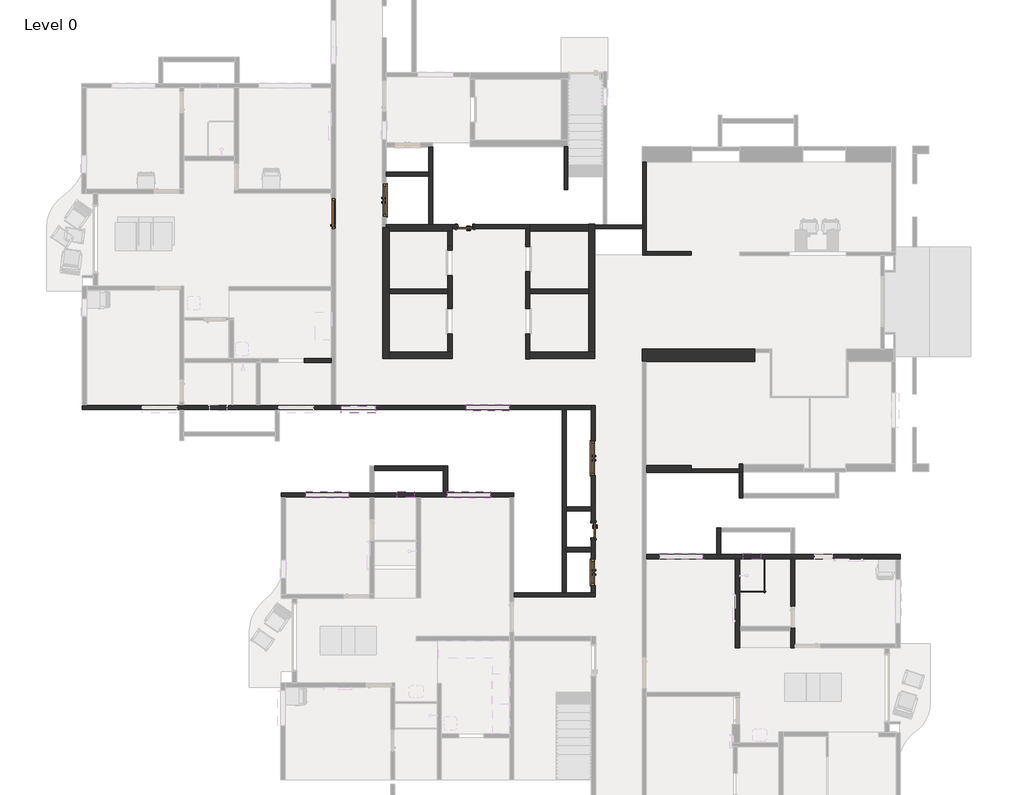
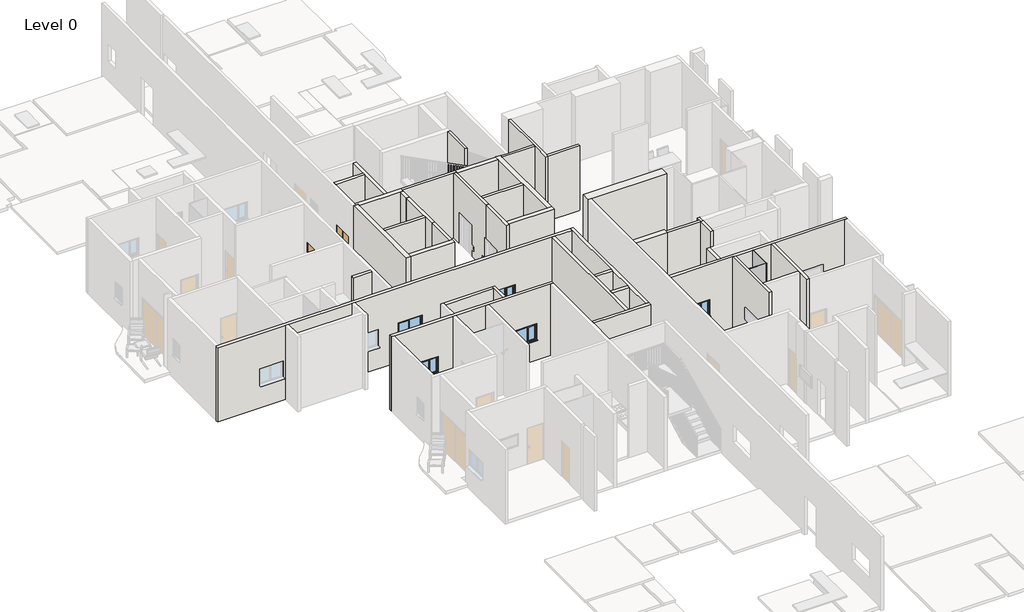
# One storey, part 5 of 14: 39 walls, 7 windows, 6 doors, 2 plates.
# Revit data of these elements (continued)
# Type "Windows_Concept_Plain_Dbl : 4'" (continued)
#   Rough Height = 910 mm
#   Height = 910 mm
#   Width = 1219.2 mm
#   Heat Transfer Coefficient (U) = 3.6886 W/(m²·K)
#   FrameOffset - External = 50 mm
#   Default Head Height = 2110 mm
#   Vis - Cavity Closers = yes
#   Define Thermal Properties by = 1
#   Material Trim = Window Frame
#   Material Glass = Glass
#   Material Frame = Window Frame
#   Wall Closure = (empty or 0)
# Type "Windows_Sgl_Plain : 2'"
#   Type Mark = "72"
#   Operation = "SinglePanel"
#   Construction Type Id = "SGL"
#   Manufacturer = "Revit"
#   Keynote = "L10"
#   Analytic Construction = "Large single-glazed windows"
#   Wrap Layers (Ext) from Ext = 102.5 mm
#   Wrap Layers (Int) from Ext = 177.5 mm
#   Window Board Projection = 25 mm
#   Window Board Extension = 25 mm
#   Visual Light Transmittance = 0.9
#   Solar Heat Gain Coefficient = 0.86
#   Rough Width = 609.6 mm
#   Rough Height = 910 mm
#   Height = 910 mm
#   Width = 609.6 mm
#   Heat Transfer Coefficient (U) = 5.5617 W/(m²·K)
#   Glazing Thickness = 24 mm
#   FrameOffset - External = 50 mm
#   Frame Depth = 65 mm
#   Default Head Height = 2110 mm
#   Cill Depth = 87.5 mm
#   Cavity Closer Width = 50 mm
#   Cavity Closer Offset from Ext = 102.5 mm
#   Cavity Closer Depth = 85 mm
#   Vis - Cavity Closers = yes
#   Define Thermal Properties by = 1
#   Material Trim = Window Frame
#   Material Glass = Glass
#   Material Frame = Window Frame
#   Wall Closure = (empty or 0)
# Type "Windows_Tpl_Variable_Casement : 5'"
#   Type Mark = "83"
#   Operation = "TriplePanelVertical"
#   Construction Type Id = "GSP4R"
#   Manufacturer = "Revit"
#   Keynote = "L10"
#   Analytic Construction = "1/8 in Pilkington single glazing"
#   Wrap Layers (Int) from Ext = 177.5 mm
#   Wrap Layers (Ext) from Ext = 102.5 mm
#   Window Board Projection = 25 mm
#   Window Board Extension = 25 mm
#   Visual Light Transmittance = 0.9
#   Solar Heat Gain Coefficient = 0.78
#   Rough Width = 1524 mm
#   Rough Height = 910 mm
#   Height = 910 mm
#   Width = 1524 mm
#   Heat Transfer Coefficient (U) = 3.6886 W/(m²·K)
#   Glazing Thickness = 24 mm
#   FrameOffset - External = 50 mm
#   Frame Depth = 65 mm
#   Default Head Height = 2110 mm
#   Cill Depth = 87.5 mm
#   Cavity Closer Width = 50 mm
#   Cavity Closer Offset from Ext = 102.5 mm
#   Cavity Closer Depth = 85 mm
#   Casement Width = 450 mm
#   Vis - Cavity Closers = yes
#   Define Thermal Properties by = 1
#   Material Trim = Window Frame
#   Material Glass = Glass
#   Material Frame = Window Frame
#   Wall Closure = (empty or 0)
# Element 1 (IfcDoor, "Doors_ExtDbl_Flush : 3'")
#   Phase Created = New Construction
#   Materials on its faces: "Door - Handle", "Door - Frame/Mullion", "Door - Panel"
# Element 2 (IfcDoor, "Doors_ExtDbl_Flush : 3.75'")
#   Phase Created = New Construction
#   Materials on its faces: "Door - Handle", "Door - Frame/Mullion", "Door - Panel"
# Element 3 (IfcDoor, "Doors_ExtDbl_Flush : 4'")
#   Phase Created = New Construction
#   Materials on its faces: "Door - Handle", "Door - Frame/Mullion", "Door - Panel"
# Element 4 (IfcDoor, "Doors_ExtSgl_Flush : D1")
#   Phase Created = New Construction
#   Materials on its faces: "Door - Handle", "Door - Frame/Mullion", "Door - Panel"
# Elements 5, 6 (IfcDoor, "Doors_IntSgl : 2'")
#   Phase Created = New Construction
#   Materials on its faces: "Door - Architrave", "Door - Handle", "Door - Frame/Mullion (1)", "Door - Panel"
# Elements 7, 8 (IfcPlate, "System Panel : Glazed")
#   Phase Created = New Construction
#   Materials on its faces: "Glass"
# Elements 9, 10, 11, 12, 13, 14, 15, 16, 17, 18, 19, 20, 21, 22, 23, 24, 25, 26, 27, 28, 29, 30, 31, 32 (IfcWall, "W1")
#   Top Offset = 0 mm
#   Base Offset = 0 mm
#   wall height = 4000 mm
#   Phase Created = New Construction
#   Base Constraint = Level 0
#   Top Constraint = Level 1
#   Materials on its faces: "Brick, Common"
# Element 33 (IfcWall, "W3")
#   Top Offset = 0 mm
#   Base Offset = 0 mm
#   wall height = 4000 mm
#   Phase Created = New Construction
#   Base Constraint = Level 0
#   Top Constraint = Level 1
#   Materials on its faces: "Brick, Common"
# Elements 34, 35, 36, 37, 38, 39 (IfcWall, "W5")
#   Top Offset = 0 mm
#   Base Offset = 0 mm
#   wall height = 4000 mm
#   Phase Created = New Construction
#   Base Constraint = Level 0
#   Top Constraint = Level 1
#   Materials on its faces: "Brick, Common"
# Elements 40, 41, 42, 43, 44, 45, 46 (IfcWall, "W6")
#   Top Offset = 0 mm
#   Base Offset = 0 mm
#   wall height = 4000 mm
#   Phase Created = New Construction
#   Base Constraint = Level 0
#   Top Constraint = Level 1
#   Materials on its faces: "Brick, Common"
# Element 47 (IfcWall, "W8")
#   Top Offset = 0 mm
#   Base Offset = 0 mm
#   wall height = 4000 mm
#   Phase Created = New Construction
#   Base Constraint = Level 0
#   Top Constraint = Level 1
#   Materials on its faces: "Brick, Common"
# Element 48 (IfcWindow, "Windows_Concept_Plain_Dbl : 4'")
#   Mark = "59"
#   Phase Created = New Construction
#   Materials on its faces: "Window Frame", "Glass"
# Element 49 (IfcWindow, "Windows_Sgl_Plain : 2'")
#   Mark = "30"
#   Phase Created = New Construction
#   Materials on its faces: "Window Frame", "Glass"
# Element 50 (IfcWindow, "Windows_Sgl_Plain : 2'")
#   Mark = "68"
#   Phase Created = New Construction
#   Materials on its faces: "Window Frame", "Glass"
# Element 51 (IfcWindow, "Windows_Tpl_Variable_Casement : 5'")
#   Mark = "28"
#   Phase Created = New Construction
#   Materials on its faces: "Window Frame", "Glass"
# Element 52 (IfcWindow, "Windows_Tpl_Variable_Casement : 5'")
#   Mark = "60"
#   Phase Created = New Construction
#   Materials on its faces: "Window Frame", "Glass"
# Element 53 (IfcWindow, "Windows_Tpl_Variable_Casement : 5'")
#   Mark = "61"
#   Phase Created = New Construction
#   Materials on its faces: "Window Frame", "Glass"
# Element 54 (IfcWindow, "Windows_Tpl_Variable_Casement : 5'")
#   Mark = "62"
#   Phase Created = New Construction
#   Materials on its faces: "Window Frame", "Glass"
# Materials
#   "Door - Panel": class "Wood", colour RGB 210 159 95, transparency 0, Keynote = "L20", Cost = 0
#   "Door - Frame/Mullion": class "Wood", colour RGB 212 179 113, transparency 0, Keynote = "L20", Cost = 0
#   "Door - Handle": colour RGB 0 0 0, transparency 0, Keynote = "P21", Cost = 0
#   "Door - Frame/Mullion (1)": class "Wood", colour RGB 212 179 113, transparency 0, Keynote = "L20", Cost = 0
#   "Door - Architrave": class "Wood", colour RGB 154 90 5, transparency 0, Keynote = "P20", Cost = 0
#   "Brick, Common": class "Masonry", colour RGB 170 100 105, transparency 0, Description = "Common brick", Cost = 0
#   "Window Frame": colour RGB 249 249 249, transparency 0, Keynote = "L10", Cost = 0
#   "Glass": class "Glass", colour RGB 0 128 192, transparency 0.9, Description = "Soda Lime Glass", Cost = 0
